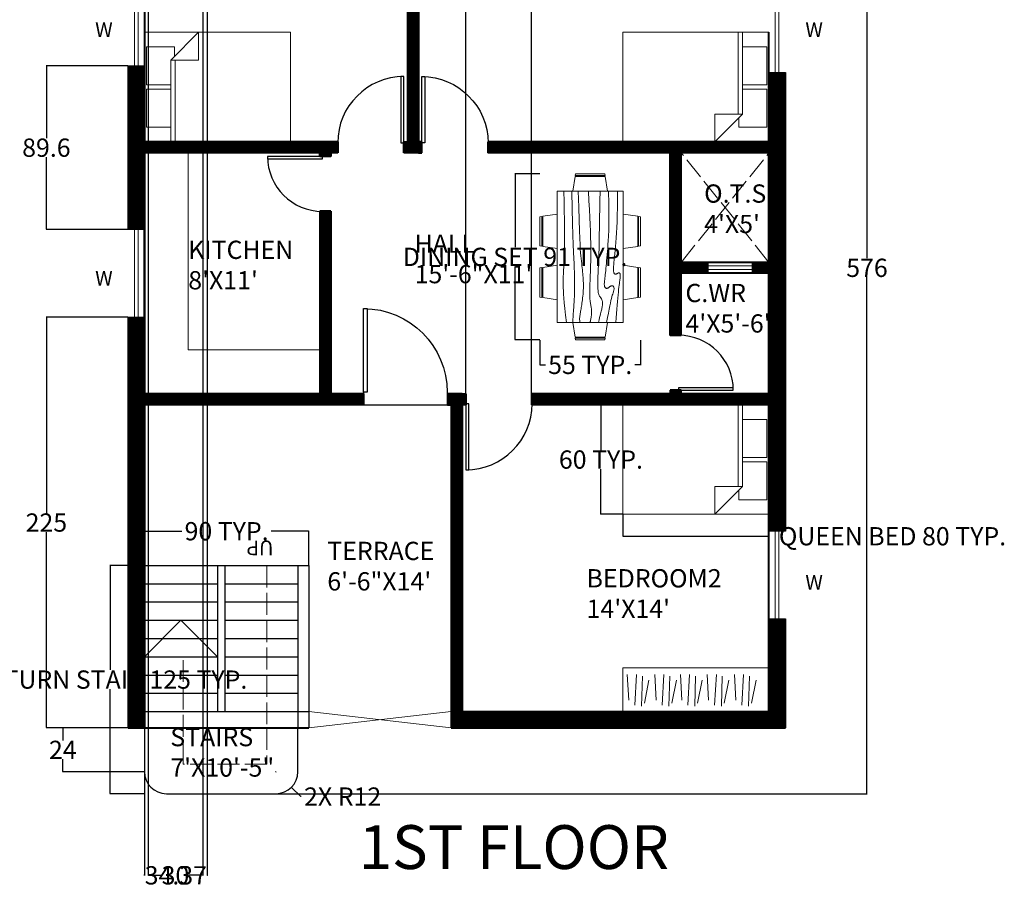
# Model space of a CAD drawing. Units: inches. Extents: x 345 to 1363, y 285 to 1014.
# Tile 3 of 4: x 824 to 1363, y 285 to 760. Entities that reach past the tile are written whole.
import ezdxf

# ---------------------------------------------------------------- set-up
doc = ezdxf.new("R2010")
doc.units = ezdxf.units.IN
doc.header["$MEASUREMENT"] = 0
doc.linetypes.add('ACAD_ISO02W100', pattern=[15, 12, -3])
for name, color, linetype, lineweight in [('A-ANNO-DIMS', 2, 'Continuous', 18), ('A-ANNO-SYMB', 3, 'Continuous', 18), ('A-ANNO-TEXT', 7, 'Continuous', 18), ('A-ANNO-TITL', 7, 'Continuous', 35), ('A-AREA-IDEN', 7, 'Continuous', 18), ('A-FLOR-CASE', 8, 'Continuous', 18), ('A-FLOR-OPEN', 8, 'Continuous', 18), ('A-FLOR-OPEN-OVHD', 8, 'ACAD_ISO02W100', 13), ('A-FLOR-STRS', 7, 'Continuous', 25), ('A-FLOR-STRS-PATH', 3, 'ACAD_ISO02W100', 18), ('A-FURN', 9, 'Continuous', 18), ('A-GLAZ', 4, 'Continuous', 18), ('A-WALL', 7, 'Continuous', 40), ('A-WALL-PATT', 252, 'Continuous', 9), ('BED', 9, 'Continuous', 18), ('DOOR', 4, 'Continuous', 25)]:
    doc.layers.add(name, color=color, linetype=linetype, lineweight=lineweight)
doc.styles.get("Standard").update_dxf_attribs({"font": 'arial.ttf'})
doc.dimstyles.get("Standard").update_dxf_attribs({"dimtxt": 10, "dimasz": 0.18, "dimexe": 0.18, "dimexo": 0.0625, "dimgap": 0.09, "dimtad": 0, "dimtih": 1, "dimtoh": 1, "dimdec": 0, "dimzin": 0, "dimdsep": 46, "dimlunit": 3, "dimtxsty": 'Standard', "dimcen": 0.09, "dimadec": 0, "dimazin": 0, "dimtfac": 1, "dimtdec": 0, "dimtofl": 0, "dimtmove": 0, "dimatfit": 3, "dimfxl": 1, "dimtolj": 1, "dimtzin": 0, "dimarcsym": 0})

# ---------------------------------------------------------------- blocks, each defined once
blk = doc.blocks.new('Bed - Queen')
for p, q in [((0, -80.00003), (0, 0)), ((0, 0), (59.99999, 0)), ((59.99999, 0), (59.99999, -80.00003)), ((7.99999, -1.2), (28.79998, -1.2)), ((7.99999, -14.4), (7.99999, -1.2)), ((28.79998, -1.2), (28.79998, -14.4)), ((31.19999, -1.2), (51.99999, -1.2)), ((31.19999, -14.4), (31.19999, -1.2)), ((51.99999, -1.2), (51.99999, -16.4)), ((0, -14.4), (44.8, -14.4)), ((59.99999, -29.6), (44.8, -14.4)), ((44.8, -14.4), (44.8, -29.6)), ((44.8, -16.8), (0, -16.8)), ((51.99999, -16.4), (46.79936, -16.4)), ((44.8, -29.6), (59.99999, -29.6)), ((59.99999, -80.00003), (0, -80.00003))]:
    blk.add_line(p, q)
blk = doc.blocks.new('Dining Set - 36 x 72 in.')
for p, q in [((-22, 27.5), (-22.1562, 26.50042)), ((-22, 27.5), (-6, 27.5)), ((-5.8437, 26.49966), (-6, 27.5)), ((6, 27.5), (5.8438, 26.50042)), ((6, 27.5), (22, 27.5)), ((22.1563, 26.49966), (22, 27.5)), ((-22.2343, 26.00059), (-23.4847, 17.99762)), ((-22.2304, 26), (-5.7608, 26)), ((-5.8416, 26.5), (-22.1534, 26.5)), ((-4.5152, 17.99762), (-5.7655, 25.99926)), ((5.7657, 26.00059), (4.5153, 17.99762)), ((5.7696, 26), (22.2392, 26)), ((22.1584, 26.5), (5.8466, 26.5)), ((23.4848, 17.99762), (22.2345, 25.99926)), ((36, 18), (-36, 18)), ((-36, 18), (-36, -18)), ((36, -18), (36, 18)), ((-45.5, 8), (-44.5004, 8.15617)), ((-45.5, 8), (-45.5, -8)), ((-44.5, -8.15843), (-44.5, 8.15338)), ((-44.0006, 8.23428), (-35.9976, 9.48474)), ((-44, 8.23041), (-44, -8.23915)), ((44.0006, 8.23428), (35.9976, 9.48474)), ((44, 8.23041), (44, -8.23915)), ((44.5, -8.15843), (44.5, 8.15338)), ((45.5, 8), (44.5005, 8.15617)), ((45.5, 8), (45.5, -8)), ((-44.4997, -8.15631), (-45.5, -8)), ((-35.9976, -9.48476), (-43.9993, -8.2345)), ((35.9976, -9.48476), (43.9993, -8.2345)), ((44.4997, -8.15631), (45.5, -8)), ((-36, -18), (36, -18)), ((-22.2343, -26.0006), (-23.4847, -17.99762)), ((-4.5152, -17.99762), (-5.7655, -25.99928)), ((5.7657, -26.0006), (4.5153, -17.99762)), ((23.4848, -17.99762), (22.2345, -25.99928)), ((-22.2304, -26), (-5.7608, -26)), ((-22, -27.5), (-22.1562, -26.50044)), ((-5.8416, -26.5), (-22.1534, -26.5)), ((-5.8437, -26.49967), (-6, -27.5)), ((5.7696, -26), (22.2392, -26)), ((6, -27.5), (5.8438, -26.50044)), ((22.1584, -26.5), (5.8466, -26.5)), ((22.1563, -26.49967), (22, -27.5)), ((-22, -27.5), (-6, -27.5)), ((6, -27.5), (22, -27.5))]:
    blk.add_line(p, q)
for points in [[(-36, 15), (-31.1772, 14.97754), (-26.8079, 14.91406), (-22.8538, 14.81543), (-19.276, 14.6875), (-16.0362, 14.53613), (-13.0957, 14.36718), (-10.4159, 14.18652), (-7.9583, 14), (-5.6904, 13.81315), (-3.6035, 13.63021), (-1.6954, 13.45508), (0.0365, 13.29166), (1.5945, 13.14388), (2.9811, 13.01562), (4.1988, 12.9108), (5.25, 12.83333), (6.1393, 12.78613), (6.8802, 12.76823), (7.4883, 12.77767), (7.9792, 12.8125), (8.3685, 12.87077), (8.6719, 12.95052), (8.9049, 13.0498), (9.0833, 13.16666), (9.2205, 13.29899), (9.3216, 13.44401), (9.3895, 13.59879), (9.4271, 13.76041), (9.4373, 13.92594), (9.4232, 14.09245), (9.3875, 14.257), (9.3333, 14.41666), (9.2638, 14.56917), (9.1836, 14.71484), (9.0975, 14.85465), (9.0104, 14.98958), (8.9272, 15.1206), (8.8529, 15.2487), (8.7922, 15.37483), (8.75, 15.5), (8.7305, 15.62467), (8.7344, 15.74739), (8.7617, 15.86621), (8.8125, 15.97916), (8.8867, 16.08431), (8.9844, 16.17968), (9.1055, 16.26334), (9.25, 16.33333), (9.4189, 16.38802), (9.6172, 16.42708), (9.8506, 16.45052), (10.125, 16.45833), (10.4463, 16.45052), (10.8203, 16.42708), (11.2529, 16.38802), (11.75, 16.33333), (12.3184, 16.26318), (12.9694, 16.17838), (13.7151, 16.07991), (14.5677, 15.96875), (15.5395, 15.84586), (16.6426, 15.71224), (17.8893, 15.56884), (19.2917, 15.41666), (20.859, 15.25667), (22.5879, 15.08984), (24.4721, 14.91715), (26.5052, 14.73958), (28.6809, 14.5581), (30.9929, 14.3737), (33.4347, 14.18733), (36, 14)], [(-36, 10), (-28.9766, 10.14274), (-23.1725, 10.20442), (-18.4241, 10.19775), (-14.5677, 10.13541), (-11.4399, 10.03011), (-8.877, 9.89453), (-6.7154, 9.74137), (-4.7917, 9.58333), (-2.9698, 9.43082), (-1.2246, 9.28515), (0.4415, 9.14534), (2.026, 9.01041), (3.5266, 8.87939), (4.9408, 8.7513), (6.266, 8.62516), (7.5, 8.5), (8.6411, 8.37549), (9.6914, 8.2539), (10.6538, 8.13818), (11.5312, 8.03125), (12.3267, 7.93603), (13.043, 7.85547), (13.6831, 7.79248), (14.25, 7.75), (14.7471, 7.7303), (15.1797, 7.73307), (15.5537, 7.75732), (15.875, 7.80208), (16.1494, 7.86637), (16.3828, 7.94922), (16.5811, 8.04964), (16.75, 8.16666), (16.8944, 8.29915), (17.0143, 8.44531), (17.1089, 8.60319), (17.1771, 8.77083), (17.218, 8.94629), (17.2305, 9.1276), (17.2137, 9.31282), (17.1667, 9.5), (17.0895, 9.6875), (16.987, 9.875), (16.8649, 10.0625), (16.7292, 10.25), (16.5856, 10.4375), (16.4401, 10.625), (16.2985, 10.8125), (16.1667, 11), (16.05, 11.18733), (15.9518, 11.3737), (15.8752, 11.5581), (15.8229, 11.73958), (15.798, 11.91715), (15.8034, 12.08984), (15.842, 12.25667), (15.9167, 12.41666), (16.0295, 12.56836), (16.1784, 12.70833), (16.3605, 12.83268), (16.5729, 12.9375), (16.8127, 13.01888), (17.0768, 13.07291), (17.3625, 13.0957), (17.6667, 13.08333), (17.9894, 13.03312), (18.3418, 12.94726), (18.7382, 12.82918), (19.1927, 12.68229), (19.7195, 12.51001), (20.3327, 12.31575), (21.0465, 12.10294), (21.875, 11.875), (22.8357, 11.63354), (23.959, 11.37304), (25.2786, 11.08618), (26.8282, 10.76562), (28.6414, 10.40405), (30.752, 9.99414), (33.1936, 9.52856), (36, 9)], [(-36, 5.5), (-30.7157, 5.3348), (-26.069, 5.20963), (-21.9946, 5.11767), (-18.4271, 5.05208), (-15.3009, 5.00602), (-12.5508, 4.97265), (-10.1112, 4.94515), (-7.9167, 4.91666), (-5.909, 4.88167), (-4.0586, 4.83984), (-2.3429, 4.79215), (-0.7396, 4.73958), (0.7739, 4.6831), (2.22, 4.6237), (3.6213, 4.56233), (5, 4.5), (6.373, 4.43782), (7.7344, 4.3776), (9.0723, 4.32129), (10.375, 4.27083), (11.6309, 4.22819), (12.8281, 4.19531), (13.9551, 4.17415), (15, 4.16666), (15.954, 4.17448), (16.819, 4.19791), (17.6001, 4.23698), (18.3021, 4.29166), (18.9299, 4.36198), (19.4883, 4.44791), (19.9823, 4.54948), (20.4167, 4.66666), (20.7969, 4.79899), (21.1302, 4.94401), (21.4245, 5.09879), (21.6875, 5.26041), (21.9271, 5.42594), (22.1511, 5.59245), (22.3672, 5.757), (22.5834, 5.91666), (22.8065, 6.06868), (23.0404, 6.21093), (23.2879, 6.34147), (23.5521, 6.45833), (23.8358, 6.55957), (24.142, 6.64323), (24.4735, 6.70735), (24.8334, 6.75), (25.2235, 6.76969), (25.642, 6.76692), (26.0858, 6.74267), (26.5521, 6.69791), (27.0379, 6.63362), (27.5404, 6.55078), (28.0565, 6.45036), (28.5834, 6.33333), (29.1242, 6.19987), (29.7071, 6.04687), (30.3661, 5.87044), (31.1354, 5.66666), (32.0493, 5.43164), (33.142, 5.16146), (34.4475, 4.85221), (36, 4.5)], [(-36, -1), (-30.7915, -0.6591), (-26.0195, -0.38216), (-21.6519, -0.16284), (-17.6563, 0.00521), (-14.0005, 0.12833), (-10.6523, 0.21289), (-7.5796, 0.26522), (-4.75, 0.29166), (-2.134, 0.29793), (0.2878, 0.28711), (2.5317, 0.26163), (4.6146, 0.22396), (6.5529, 0.17651), (8.3633, 0.12174), (10.0623, 0.06209), (11.6667, 0), (13.1899, -0.06201), (14.6341, -0.1211), (15.9982, -0.17432), (17.2813, -0.21875), (18.4823, -0.25147), (19.6003, -0.26953), (20.6343, -0.27002), (21.5834, -0.25), (22.4481, -0.20768), (23.2357, -0.14584), (23.9549, -0.06836), (24.6146, 0.02083), (25.2235, 0.11784), (25.7904, 0.21875), (26.3241, 0.31966), (26.8334, 0.41666), (27.3265, 0.50618), (27.8099, 0.58593), (28.2894, 0.65397), (28.7709, 0.70833), (29.2601, 0.74707), (29.763, 0.76823), (30.2855, 0.76985), (30.8334, 0.75), (31.4088, 0.70784), (31.9994, 0.64713), (32.589, 0.57275), (33.1615, 0.48958), (33.7008, 0.4025), (34.1908, 0.3164), (34.6153, 0.23616), (34.9584, 0.16666), (35.2099, 0.11165), (35.3848, 0.07031), (35.504, 0.04069), (35.5886, 0.02083), (35.6594, 0.00879), (35.7377, 0.0026), (35.8442, 0.00032), (36, 0)], [(-36, -6.5), (-27.1843, -6.31267), (-20.084, -6.1263), (-14.469, -5.9419), (-10.1094, -5.76042), (-6.7752, -5.58285), (-4.2363, -5.41016), (-2.2629, -5.24333), (-0.625, -5.08334), (0.8708, -4.93099), (2.2715, -4.78646), (3.5872, -4.64974), (4.8281, -4.52084), (6.0046, -4.39974), (7.127, -4.28646), (8.2053, -4.18099), (9.25, -4.08334), (10.2705, -3.99382), (11.2734, -3.91407), (12.2647, -3.84603), (13.25, -3.79167), (14.2354, -3.75293), (15.2266, -3.73177), (16.2295, -3.73015), (17.25, -3.75), (18.2912, -3.79248), (19.3451, -3.85547), (20.4009, -3.93604), (21.4479, -4.03125), (22.4754, -4.13819), (23.4727, -4.25391), (24.4289, -4.37549), (25.3334, -4.5), (26.1785, -4.62492), (26.9694, -4.74935), (27.7145, -4.87281), (28.4219, -4.99479), (29.1, -5.11483), (29.7572, -5.23242), (30.4016, -5.34709), (31.0417, -5.45834), (31.6837, -5.56437), (32.3262, -5.65821), (32.9658, -5.73153), (33.599, -5.77604), (34.2224, -5.78345), (34.8327, -5.74545), (35.4264, -5.65373), (36, -5.5)], [(-36, -10), (-26.4022, -9.81299), (-18.4675, -9.62891), (-11.9839, -9.45069), (-6.7396, -9.28125), (-2.5226, -9.12354), (0.8789, -8.98047), (3.6769, -8.85498), (6.0833, -8.75), (8.2767, -8.66765), (10.3021, -8.60677), (12.1712, -8.56543), (13.8958, -8.54167), (15.4876, -8.53353), (16.9583, -8.53907), (18.3197, -8.55632), (19.5834, -8.58334), (20.7616, -8.61841), (21.8685, -8.66081), (22.9188, -8.71004), (23.9271, -8.76563), (24.9081, -8.82707), (25.8763, -8.89388), (26.8465, -8.96558), (27.8334, -9.04167), (28.8474, -9.12118), (29.8828, -9.20117), (30.93, -9.27824), (31.9792, -9.34896), (33.0205, -9.40991), (34.0443, -9.45768), (35.0407, -9.48885), (36, -9.5)], [(-36, -14.5), (-30.0881, -14.33513), (-25.0332, -14.21224), (-20.7312, -14.12647), (-17.0781, -14.07292), (-13.97, -14.04671), (-11.3027, -14.04297), (-8.9724, -14.05681), (-6.875, -14.08334), (-4.9224, -14.11833), (-3.0905, -14.16016), (-1.3709, -14.20785), (0.2448, -14.26042), (1.7647, -14.3169), (3.1973, -14.3763), (4.5507, -14.43767), (5.8333, -14.5), (7.0554, -14.5621), (8.235, -14.62175), (9.3922, -14.67652), (10.5469, -14.72396), (11.7192, -14.76164), (12.929, -14.78711), (14.1965, -14.79794), (15.5417, -14.79167), (16.9933, -14.76424), (18.6152, -14.70508), (20.4804, -14.60197), (22.6615, -14.44271), (25.2312, -14.21509), (28.2624, -13.9069), (31.8277, -13.50594), (36, -13)]]:
    blk.add_lwpolyline(points)
blk = doc.blocks.new('*U8')
for p, q in [((0, 0), (0, -6)), ((-40, 0), (-40, -6))]:
    blk.add_line(p, q)
blk.add_lwpolyline([(0, 0), (0, 40), (-1.75, 40), (-1.75, 0)], close=True)
blk.add_arc((0, 0), 40, 90, 180)
blk = doc.blocks.new('*U9')
for p, q in [((0, 0), (0, 6)), ((40, 0), (40, 6))]:
    blk.add_line(p, q)
blk.add_lwpolyline([(0, 0), (0, -40), (1.75, -40), (1.75, 0)], close=True)
blk.add_arc((0, 0), 40, 270, 360)
blk = doc.blocks.new('WIN-48IN-EXT')
for p, q in [((9, 48), (0, 48)), ((3.5, 0), (3.5, 48)), ((5.5, 0), (5.5, 48)), ((9, 0), (0, 0))]:
    blk.add_line(p, q)
blk = doc.blocks.new('WIN-24IN-VENT')
for p, q in [((0, 24), (6, 24)), ((2, 24), (2, 0)), ((4, 24), (4, 0)), ((0, 0), (6, 0))]:
    blk.add_line(p, q)
blk = doc.blocks.new('WARDROBE-80X24')
for p, q in [((0, 0), (0, 24)), ((80, 0), (80, 24)), ((2.45, 20.28), (3.21, 6.18)), ((7.49, 20.28), (6.48, 3.41)), ((10.77, 19.28), (10.26, 2.91)), ((14.3, 17.26), (11.77, 4.67)), ((17.45, 20.28), (18.2, 6.18)), ((22.49, 20.28), (21.48, 3.41)), ((25.77, 19.28), (25.26, 2.91)), ((29.29, 17.26), (26.77, 4.67)), ((31.55, 20.28), (32.31, 6.18)), ((36.59, 20.28), (35.59, 3.41)), ((39.87, 19.28), (39.37, 2.91)), ((43.4, 17.26), (40.88, 4.67)), ((46.16, 20.28), (46.91, 6.18)), ((51.2, 20.28), (50.19, 3.41)), ((54.47, 19.28), (53.97, 2.91)), ((58, 17.26), (55.48, 4.67)), ((61.07, 20.28), (61.83, 6.18)), ((66.11, 20.28), (65.1, 3.41)), ((69.39, 19.28), (68.88, 2.91)), ((72.92, 17.26), (70.4, 4.67)), ((80, 0), (0, 0))]:
    blk.add_line(p, q)
blk = doc.blocks.new('KITCHEN-L-COUNTER')
for p in [(0, 108), (72, 0)]:
    blk.add_line(p, (0, 0))
blk = doc.blocks.new('STAIR-RETURN-84IN')
for p, q in [((0, 89), (44, 89)), ((40, 89), (40, 9)), ((44, 89), (44, 9)), ((44, 89), (90, 89)), ((84, 89), (84, 0)), ((90, 89), (90, 0)), ((0, 79), (40, 79)), ((44, 79), (84, 79)), ((0, 69), (40, 69)), ((44, 69), (84, 69)), ((0, 59), (40, 59)), ((44, 59), (84, 59)), ((0, 49), (40, 49)), ((44, 49), (84, 49)), ((0, 39), (40, 39)), ((44, 39), (84, 39)), ((0, 29), (40, 29)), ((44, 29), (84, 29)), ((0, 19), (40, 19)), ((44, 19), (84, 19)), ((0, 9), (90, 9)), ((0, 0), (0, -24)), ((84, -24), (84, 0)), ((12, -36), (72, -36))]:
    blk.add_line(p, q)
for centre, start, end in [((12, -24), 180, 270), ((72, -24), 270, 0)]:
    blk.add_arc(centre, 12, start, end)
blk = doc.blocks.new('STAIR-DIRECTION-ARROWHEAD')
for p, q in [((-20, 0), (0, 20)), ((0, 20), (20, 0)), ((0, 0), (-20, 0)), ((20, 0), (1.17, 0))]:
    blk.add_line(p, q)
blk = doc.blocks.new('*D20')
at = {"layer": 'A-ANNO-DIMS', "color": 0, "lineweight": -2, "transparency": 16777216}
for p, q in [((1154.38, 488.7), (1154.38, 476.58)), ((1234.38, 488.7), (1234.38, 476.58)), ((1154.56, 476.76), (1234.2, 476.76)), ((1234.38, 476.76), (1234.56, 476.76))]:
    blk.add_line(p, q, dxfattribs=at)
at = {"layer": 'A-ANNO-DIMS', "color": 0, "transparency": 16777216}
for points in [[(1154.56, 476.79), (1154.56, 476.73), (1154.38, 476.76)], [(1234.2, 476.79), (1234.2, 476.73), (1234.38, 476.76)]]:
    blk.add_solid(points, dxfattribs=at)
at = {"layer": 'Defpoints', "color": 0, "transparency": 16777216}
for p in [(1154.38, 488.76), (1234.38, 488.76), (1234.38, 476.76)]:
    blk.add_point(p, dxfattribs=at)
at = {"layer": 'A-ANNO-DIMS', "color": 0, "transparency": 16777216, "insert": (1302.06, 476.76), "char_height": 10, "attachment_point": 5}
blk.add_mtext('\\A1;QUEEN BED 80 TYP.', dxfattribs=at)
blk = doc.blocks.new('*D21')
at = {"layer": 'A-ANNO-DIMS', "color": 0, "lineweight": -2, "transparency": 16777216}
for p, q in [((1154.32, 548.76), (1142.2, 548.76)), ((1142.38, 548.58), (1142.38, 523.96)), ((1142.38, 488.94), (1142.38, 513.57)), ((1154.32, 488.76), (1142.2, 488.76))]:
    blk.add_line(p, q, dxfattribs=at)
at = {"layer": 'A-ANNO-DIMS', "color": 0, "transparency": 16777216}
for points in [[(1142.35, 548.58), (1142.41, 548.58), (1142.38, 548.76)], [(1142.35, 488.94), (1142.41, 488.94), (1142.38, 488.76)]]:
    blk.add_solid(points, dxfattribs=at)
at = {"layer": 'Defpoints', "color": 0, "transparency": 16777216}
for p in [(1154.38, 548.76), (1142.38, 488.76), (1154.38, 488.76)]:
    blk.add_point(p, dxfattribs=at)
at = {"layer": 'A-ANNO-DIMS', "color": 0, "transparency": 16777216, "insert": (1142.38, 518.76), "char_height": 10, "attachment_point": 5}
blk.add_mtext('\\A1;60 TYP.', dxfattribs=at)
blk = doc.blocks.new('*D24')
at = {"layer": 'A-ANNO-DIMS', "color": 0, "lineweight": -2, "transparency": 16777216}
for p, q in [((1108.94, 675.25), (1095.17, 675.25)), ((1095.35, 675.07), (1095.35, 635.01)), ((1095.35, 584.43), (1095.35, 624.48)), ((1108.94, 584.25), (1095.17, 584.25))]:
    blk.add_line(p, q, dxfattribs=at)
at = {"layer": 'A-ANNO-DIMS', "color": 0, "transparency": 16777216}
for points in [[(1095.32, 675.07), (1095.38, 675.07), (1095.35, 675.25)], [(1095.32, 584.43), (1095.38, 584.43), (1095.35, 584.25)]]:
    blk.add_solid(points, dxfattribs=at)
at = {"layer": 'Defpoints', "color": 0, "transparency": 16777216}
for p in [(1109, 675.25), (1095.35, 584.25), (1109, 584.25)]:
    blk.add_point(p, dxfattribs=at)
at = {"layer": 'A-ANNO-DIMS', "color": 0, "transparency": 16777216, "insert": (1095.35, 629.75), "char_height": 10, "attachment_point": 5}
blk.add_mtext('\\A1;DINING SET 91 TYP.', dxfattribs=at)
blk = doc.blocks.new('*D25')
at = {"layer": 'A-ANNO-DIMS', "color": 0, "lineweight": -2, "transparency": 16777216}
for p, q in [((1109, 584.18), (1109, 570.42)), ((1164, 584.18), (1164, 570.42)), ((1109.18, 570.6), (1112.07, 570.6)), ((1163.82, 570.6), (1160.93, 570.6))]:
    blk.add_line(p, q, dxfattribs=at)
at = {"layer": 'A-ANNO-DIMS', "color": 0, "transparency": 16777216}
for points in [[(1109.18, 570.63), (1109.18, 570.57), (1109, 570.6)], [(1163.82, 570.63), (1163.82, 570.57), (1164, 570.6)]]:
    blk.add_solid(points, dxfattribs=at)
at = {"layer": 'Defpoints', "color": 0, "transparency": 16777216}
for p in [(1109, 584.25), (1164, 584.25), (1164, 570.6)]:
    blk.add_point(p, dxfattribs=at)
at = {"layer": 'A-ANNO-DIMS', "color": 0, "transparency": 16777216, "insert": (1136.5, 570.6), "char_height": 10, "attachment_point": 5}
blk.add_mtext('\\A1;55 TYP.', dxfattribs=at)
blk = doc.blocks.new('*D28')
at = {"layer": 'A-ANNO-DIMS', "color": 0, "lineweight": -2, "transparency": 16777216}
for p, q in [((892.32, 460.76), (873.45, 460.76)), ((873.63, 460.58), (873.63, 403.52)), ((873.63, 335.94), (873.63, 393)), ((892.32, 335.76), (873.45, 335.76))]:
    blk.add_line(p, q, dxfattribs=at)
at = {"layer": 'A-ANNO-DIMS', "color": 0, "transparency": 16777216}
for points in [[(873.6, 460.58), (873.66, 460.58), (873.63, 460.76)], [(873.6, 335.94), (873.66, 335.94), (873.63, 335.76)]]:
    blk.add_solid(points, dxfattribs=at)
at = {"layer": 'Defpoints', "color": 0, "transparency": 16777216}
for p in [(873.63, 460.76), (892.38, 460.76), (892.38, 335.76)]:
    blk.add_point(p, dxfattribs=at)
at = {"layer": 'A-ANNO-DIMS', "color": 0, "transparency": 16777216, "insert": (873.63, 398.26), "char_height": 10, "attachment_point": 5}
blk.add_mtext('\\A1;RETURN STAIR 125 TYP.', dxfattribs=at)
blk = doc.blocks.new('*D29')
at = {"layer": 'A-ANNO-DIMS', "color": 0, "lineweight": -2, "transparency": 16777216}
for p, q in [((892.38, 460.83), (892.38, 479.69)), ((892.56, 479.51), (912.95, 479.51)), ((982.2, 479.51), (961.81, 479.51)), ((982.38, 460.83), (982.38, 479.69))]:
    blk.add_line(p, q, dxfattribs=at)
at = {"layer": 'A-ANNO-DIMS', "color": 0, "transparency": 16777216}
for points in [[(892.56, 479.54), (892.56, 479.48), (892.38, 479.51)], [(982.2, 479.54), (982.2, 479.48), (982.38, 479.51)]]:
    blk.add_solid(points, dxfattribs=at)
at = {"layer": 'Defpoints', "color": 0, "transparency": 16777216}
for p in [(982.38, 479.51), (892.38, 460.76), (982.38, 460.76)]:
    blk.add_point(p, dxfattribs=at)
at = {"layer": 'A-ANNO-DIMS', "color": 0, "transparency": 16777216, "insert": (937.38, 479.51), "char_height": 10, "attachment_point": 5}
blk.add_mtext('\\A1;90 TYP.', dxfattribs=at)
blk = doc.blocks.new('*D33')
at = {"layer": 'A-ANNO-DIMS', "color": 0, "lineweight": -2, "transparency": 16777216}
for p, q in [((1243.44, 911.76), (1288.26, 911.76)), ((1288.08, 911.58), (1288.08, 628.96)), ((1288.08, 335.94), (1288.08, 618.57)), ((964.44, 335.76), (1288.26, 335.76))]:
    blk.add_line(p, q, dxfattribs=at)
at = {"layer": 'A-ANNO-DIMS', "color": 0, "transparency": 16777216}
for points in [[(1288.05, 911.58), (1288.11, 911.58), (1288.08, 911.76)], [(1288.05, 335.94), (1288.11, 335.94), (1288.08, 335.76)]]:
    blk.add_solid(points, dxfattribs=at)
at = {"layer": 'Defpoints', "color": 0, "transparency": 16777216}
for p in [(1243.38, 911.76), (1288.08, 911.76), (964.38, 335.76)]:
    blk.add_point(p, dxfattribs=at)
at = {"layer": 'A-ANNO-DIMS', "color": 0, "transparency": 16777216, "insert": (1288.08, 623.76), "char_height": 10, "attachment_point": 5}
blk.add_mtext('\\A1;576', dxfattribs=at)
blk = doc.blocks.new('*D34')
at = {"layer": 'A-ANNO-DIMS', "color": 0, "lineweight": -2, "transparency": 16777216}
for p, q in [((883.32, 596.76), (838.5, 596.76)), ((838.68, 596.58), (838.68, 489.46)), ((838.68, 371.94), (838.68, 479.07)), ((883.32, 371.76), (838.5, 371.76))]:
    blk.add_line(p, q, dxfattribs=at)
at = {"layer": 'A-ANNO-DIMS', "color": 0, "transparency": 16777216}
for points in [[(838.65, 596.58), (838.71, 596.58), (838.68, 596.76)], [(838.65, 371.94), (838.71, 371.94), (838.68, 371.76)]]:
    blk.add_solid(points, dxfattribs=at)
at = {"layer": 'Defpoints', "color": 0, "transparency": 16777216}
for p in [(838.68, 596.76), (883.38, 596.76), (883.38, 371.76)]:
    blk.add_point(p, dxfattribs=at)
at = {"layer": 'A-ANNO-DIMS', "color": 0, "transparency": 16777216, "insert": (838.68, 484.26), "char_height": 10, "attachment_point": 5}
blk.add_mtext('\\A1;225', dxfattribs=at)
blk = doc.blocks.new('*D35')
at = {"layer": 'A-ANNO-DIMS', "color": 0, "lineweight": -2, "transparency": 16777216}
for p, q in [((883.32, 734.36), (838.5, 734.36)), ((838.68, 734.18), (838.68, 694.76)), ((838.68, 644.94), (838.68, 684.37)), ((883.32, 644.76), (838.5, 644.76))]:
    blk.add_line(p, q, dxfattribs=at)
at = {"layer": 'A-ANNO-DIMS', "color": 0, "transparency": 16777216}
for points in [[(838.65, 734.18), (838.71, 734.18), (838.68, 734.36)], [(838.65, 644.94), (838.71, 644.94), (838.68, 644.76)]]:
    blk.add_solid(points, dxfattribs=at)
at = {"layer": 'Defpoints', "color": 0, "transparency": 16777216}
for p in [(838.68, 734.36), (883.38, 734.36), (883.38, 644.76)]:
    blk.add_point(p, dxfattribs=at)
at = {"layer": 'A-ANNO-DIMS', "color": 0, "transparency": 16777216, "insert": (838.68, 689.56), "char_height": 10, "attachment_point": 5}
blk.add_mtext('\\A1;89.6', dxfattribs=at)
blk = doc.blocks.new('*D36')
at = {"layer": 'A-ANNO-DIMS', "color": 0, "lineweight": -2, "transparency": 16777216}
for p, q in [((892.32, 371.76), (847.5, 371.76)), ((847.68, 371.58), (847.68, 364.87)), ((847.68, 347.94), (847.68, 354.65)), ((892.32, 347.76), (847.5, 347.76))]:
    blk.add_line(p, q, dxfattribs=at)
at = {"layer": 'A-ANNO-DIMS', "color": 0, "transparency": 16777216}
for points in [[(847.65, 371.58), (847.71, 371.58), (847.68, 371.76)], [(847.65, 347.94), (847.71, 347.94), (847.68, 347.76)]]:
    blk.add_solid(points, dxfattribs=at)
at = {"layer": 'Defpoints', "color": 0, "transparency": 16777216}
for p in [(847.68, 371.76), (892.38, 371.76), (892.38, 347.76)]:
    blk.add_point(p, dxfattribs=at)
at = {"layer": 'A-ANNO-DIMS', "color": 0, "transparency": 16777216, "insert": (847.68, 359.76), "char_height": 10, "attachment_point": 5}
blk.add_mtext('\\A1;24', dxfattribs=at)
blk = doc.blocks.new('*D41')
at = {"layer": 'A-ANNO-DIMS', "color": 0, "lineweight": -2, "transparency": 16777216}
for p, q in [((894.38, 824.7), (894.38, 290.88)), ((924.38, 824.7), (924.38, 290.88)), ((894.56, 291.06), (902.15, 291.06)), ((924.2, 291.06), (916.61, 291.06))]:
    blk.add_line(p, q, dxfattribs=at)
at = {"layer": 'A-ANNO-DIMS', "color": 0, "transparency": 16777216}
for points in [[(894.56, 291.09), (894.56, 291.03), (894.38, 291.06)], [(924.2, 291.09), (924.2, 291.03), (924.38, 291.06)]]:
    blk.add_solid(points, dxfattribs=at)
at = {"layer": 'Defpoints', "color": 0, "transparency": 16777216}
for p in [(894.38, 824.76), (924.38, 824.76), (924.38, 291.06)]:
    blk.add_point(p, dxfattribs=at)
at = {"layer": 'A-ANNO-DIMS', "color": 0, "transparency": 16777216, "insert": (909.38, 291.06), "char_height": 10, "attachment_point": 5}
blk.add_mtext('\\A1;30', dxfattribs=at)
blk = doc.blocks.new('*D42')
at = {"layer": 'A-ANNO-DIMS', "color": 0, "lineweight": -2, "transparency": 16777216}
for p, q in [((1068.38, 554.83), (1068.38, 1007.64)), ((1068.56, 1007.46), (1079.14, 1007.46)), ((1104.2, 1007.46), (1093.63, 1007.46)), ((1104.38, 554.83), (1104.38, 1007.64))]:
    blk.add_line(p, q, dxfattribs=at)
at = {"layer": 'A-ANNO-DIMS', "color": 0, "transparency": 16777216}
for points in [[(1068.56, 1007.49), (1068.56, 1007.43), (1068.38, 1007.46)], [(1104.2, 1007.49), (1104.2, 1007.43), (1104.38, 1007.46)]]:
    blk.add_solid(points, dxfattribs=at)
at = {"layer": 'Defpoints', "color": 0, "transparency": 16777216}
for p in [(1104.38, 1007.46), (1068.38, 554.76), (1104.38, 554.76)]:
    blk.add_point(p, dxfattribs=at)
at = {"layer": 'A-ANNO-DIMS', "color": 0, "transparency": 16777216, "insert": (1086.38, 1007.46), "char_height": 10, "attachment_point": 5}
blk.add_mtext('\\A1;36', dxfattribs=at)
blk = doc.blocks.new('*D46')
at = {"layer": 'A-ANNO-DIMS', "color": 0, "lineweight": -2, "transparency": 16777216}
for p, q in [((892.381853, 902.701559), (892.381853, 290.884059)), ((926.755051, 894.701559), (926.755051, 290.884059)), ((892.201853, 291.064059), (892.021853, 291.064059)), ((926.935051, 291.064059), (927.115051, 291.064059))]:
    blk.add_line(p, q, dxfattribs=at)
at = {"layer": 'A-ANNO-DIMS', "color": 0, "transparency": 16777216}
for points in [[(892.201853, 291.094059), (892.201853, 291.034059), (892.381853, 291.064059)], [(926.935051, 291.094059), (926.935051, 291.034059), (926.755051, 291.064059)]]:
    blk.add_solid(points, dxfattribs=at)
at = {"layer": 'Defpoints', "color": 0, "transparency": 16777216}
for p in [(892.381853, 902.764059), (926.755051, 894.764059), (926.755051, 291.064059)]:
    blk.add_point(p, dxfattribs=at)
at = {"layer": 'A-ANNO-DIMS', "color": 0, "transparency": 16777216, "insert": (909.568452, 291.064059), "char_height": 10, "attachment_point": 5}
blk.add_mtext('\\A1;34.37', dxfattribs=at)
blk = doc.blocks.new('*D48')
at = {"layer": 'A-ANNO-DIMS', "color": 0, "lineweight": -2, "transparency": 16777216}
for p, q in [((964.29, 347.76), (964.47, 347.76)), ((964.38, 347.67), (964.38, 347.85)), ((977.96, 334.19), (972.99, 339.15)), ((978.14, 334.19), (977.96, 334.19))]:
    blk.add_line(p, q, dxfattribs=at)
at = {"layer": 'A-ANNO-DIMS', "color": 0, "transparency": 16777216}
blk.add_solid([(973.02, 339.17), (972.97, 339.13), (972.87, 339.28)], dxfattribs=at)
at = {"layer": 'Defpoints', "color": 0, "transparency": 16777216}
for p in [(964.38, 347.76), (972.87, 339.28)]:
    blk.add_point(p, dxfattribs=at)
at = {"layer": 'A-ANNO-DIMS', "color": 0, "transparency": 16777216, "insert": (1000.95, 334.19), "char_height": 10, "attachment_point": 5}
blk.add_mtext('\\A1;2X R12', dxfattribs=at)

msp = doc.modelspace()

# ---------------------------------------------------------------- hatches: boundary and pattern name
at = {"layer": 'A-WALL-PATT'}
h = msp.add_hatch(dxfattribs=at)
h.set_pattern_fill('ANSI31', color=256)
h.paths.add_polyline_path([(760.967, 730.806), (751.967, 730.806), (751.967, 692.764), (671.967, 692.764), (598.143, 692.764), (598.143, 686.764), (697.967, 686.764), (697.967, 586.835), (702.4, 586.835, -0.0130342), (703.967, 586.794), (703.967, 686.764), (751.967, 686.764), (751.967, 626.764), (742.74, 626.764), (742.74, 620.764), (751.967, 620.764), (751.967, 554.764), (703.967, 554.764), (703.967, 556.764), (702.4, 556.764), (697.967, 556.764), (697.967, 554.764), (622.228, 554.764), (622.228, 548.764), (751.967, 548.764), (751.967, 479.508), (760.967, 479.508)])
h.paths.add_polyline_path([(760.967, 431.508), (751.967, 431.508), (751.967, 380.764), (583.967, 380.764), (583.967, 548.764), (585.967, 548.764), (585.967, 549.325), (585.967, 554.764), (583.967, 554.764), (577.967, 554.764), (575.967, 554.764), (575.967, 548.764), (577.967, 548.764), (577.967, 371.764), (760.967, 371.764)])
h.paths.add_polyline_path([(409.967, 548.764), (529.967, 548.764), (529.967, 554.764), (511.967, 554.764), (511.967, 654.693), (507.456, 654.693, -0.0123881), (505.967, 654.73), (505.967, 554.764), (409.967, 554.764), (409.967, 596.764), (400.967, 596.764), (400.967, 371.764), (409.967, 371.764)])
h.paths.add_polyline_path([(409.967, 686.764), (505.967, 686.764), (505.967, 684.764), (507.456, 684.764), (511.967, 684.764), (511.967, 686.764), (515.791, 686.764), (515.791, 692.764), (409.967, 692.764), (409.967, 734.364), (400.967, 734.364), (400.967, 644.764), (409.967, 644.764)])
h.paths.add_polyline_path([(559.967, 824.764), (561.801, 824.764), (561.801, 829.275), (561.801, 830.764), (559.967, 830.764), (559.967, 902.764), (637.967, 902.764), (637.967, 878.764), (643.967, 878.764), (643.967, 902.764), (751.967, 902.764), (751.967, 830.764), (749.967, 830.764), (749.967, 829.275), (749.967, 824.764), (751.967, 824.764), (751.967, 778.806), (760.967, 778.806), (760.967, 911.764), (400.967, 911.764), (400.967, 782.364), (409.967, 782.364), (409.967, 824.764), (411.967, 824.764), (411.967, 829.275), (411.967, 830.764), (409.967, 830.764), (409.967, 902.764), (553.967, 902.764), (553.967, 830.764), (552.038, 830.764), (552.038, 829.275), (552.038, 824.764), (553.967, 824.764), (553.967, 692.764), (552.052, 692.764), (552.052, 692.203), (552.052, 686.764), (553.967, 686.764), (559.967, 686.764), (561.882, 686.764), (561.882, 692.764), (559.967, 692.764)])
h.paths.add_polyline_path([(718.74, 626.764), (703.967, 626.764), (703.967, 620.764), (718.74, 620.764)], flags=17)
h.paths.add_polyline_path([(892.382, 824.764), (894.382, 824.764), (894.382, 829.275), (894.382, 830.764), (892.382, 830.764), (892.382, 902.764), (1036.382, 902.764), (1036.382, 830.764), (1034.453, 830.764), (1034.453, 829.275), (1034.453, 824.764), (1036.382, 824.764), (1036.382, 692.764), (1034.467, 692.764), (1034.467, 692.203), (1034.467, 686.764), (1036.382, 686.764), (1042.382, 686.764), (1044.297, 686.764), (1044.297, 692.764), (1042.382, 692.764), (1042.382, 824.764), (1044.216, 824.764), (1044.216, 829.275), (1044.216, 830.764), (1042.382, 830.764), (1042.382, 902.764), (1120.382, 902.764), (1120.382, 878.764), (1126.382, 878.764), (1126.382, 902.764), (1234.382, 902.764), (1234.382, 830.764), (1232.382, 830.764), (1232.382, 829.275), (1232.382, 824.764), (1234.382, 824.764), (1234.382, 778.806), (1243.382, 778.806), (1243.382, 911.764), (883.382, 911.764), (883.382, 782.364), (892.382, 782.364)])
h.paths.add_polyline_path([(1243.382, 730.806), (1234.382, 730.806), (1234.382, 692.764), (1080.382, 692.764), (1080.382, 686.764), (1180.382, 686.764), (1180.382, 586.764), (1186.382, 586.764), (1186.382, 686.764), (1234.382, 686.764), (1234.382, 626.764), (1225.155, 626.764), (1225.155, 620.764), (1234.382, 620.764), (1234.382, 554.764), (1186.382, 554.764), (1186.382, 556.764), (1180.382, 556.764), (1180.382, 554.764), (1104.382, 554.764), (1104.382, 548.764), (1234.382, 548.764), (1234.382, 479.508), (1243.382, 479.508)])
h.paths.add_polyline_path([(892.382, 686.764), (988.382, 686.764), (988.382, 684.764), (989.871, 684.764), (994.382, 684.764), (994.382, 686.764), (998.206, 686.764), (998.206, 692.203, -0.0038664), (998.21, 692.764), (892.382, 692.764), (892.382, 734.364), (883.382, 734.364), (883.382, 644.764), (892.382, 644.764)])
h.paths.add_polyline_path([(1066.382, 548.764), (1068.382, 548.764), (1068.382, 554.764), (1066.382, 554.764), (1060.382, 554.764), (1058.382, 554.764), (1058.382, 548.764), (1060.382, 548.764), (1060.382, 371.764), (1243.382, 371.764), (1243.382, 431.508), (1234.382, 431.508), (1234.382, 380.764), (1154.382, 380.764), (1066.382, 380.764)])
h.paths.add_polyline_path([(1201.155, 626.764), (1186.382, 626.764), (1186.382, 620.764), (1201.155, 620.764)], flags=17)
h.paths.add_polyline_path([(892.382, 596.764), (883.382, 596.764), (883.382, 371.764), (892.382, 371.764), (892.382, 548.764), (1012.382, 548.764), (1012.382, 554.764), (994.382, 554.764), (994.382, 654.764), (988.382, 654.764), (988.382, 554.764), (892.382, 554.764)])

# ---------------------------------------------------------------- linework, layer by layer
at = {"layer": 'A-FLOR-CASE'}
msp.add_line((1154.382, 404.764), (1234.382, 404.764), dxfattribs=at)
at = {"layer": 'A-FLOR-OPEN'}
for p, q in [((982.382, 380.764), (1060.382, 371.764)), ((1060.382, 380.764), (982.382, 371.764))]:
    msp.add_line(p, q, dxfattribs=at)
at = {"layer": 'A-FLOR-OPEN-OVHD'}
for p, q in [((1186.382, 626.764), (1234.382, 686.764)), ((1234.382, 626.764), (1186.382, 686.764))]:
    msp.add_line(p, q, dxfattribs=at)
at = {"layer": 'A-FLOR-STRS-PATH'}
for p, q in [((959.382, 460.764), (959.382, 371.764)), ((913.551, 351.941), (913.551, 410.764)), ((959.382, 371.764), (959.382, 351.941)), ((959.382, 351.941), (913.551, 351.941))]:
    msp.add_line(p, q, dxfattribs=at)
at = {"layer": 'A-WALL'}
for p, q in [((892.382, 824.764), (892.382, 692.764)), ((1036.382, 824.764), (1036.382, 692.764)), ((1042.382, 824.764), (1042.382, 692.764)), ((1234.382, 692.764), (1234.382, 752.764)), ((883.382, 734.364), (883.382, 644.764)), ((1243.382, 479.508), (1243.382, 730.806)), ((998.382, 692.764), (892.382, 692.764)), ((998.382, 692.764), (998.382, 686.764)), ((1034.382, 686.764), (1034.382, 692.764)), ((1034.382, 692.764), (1036.382, 692.764)), ((1044.382, 692.764), (1042.382, 692.764)), ((1044.382, 686.764), (1044.382, 692.764)), ((1234.382, 692.764), (1080.382, 692.764)), ((1080.382, 692.764), (1080.382, 686.764)), ((988.382, 686.764), (892.382, 686.764)), ((892.382, 686.764), (892.382, 554.764)), ((892.382, 554.764), (892.382, 686.764)), ((988.382, 684.764), (988.382, 686.764)), ((998.382, 686.764), (994.382, 686.764)), ((994.382, 686.764), (994.382, 684.764)), ((1036.382, 686.764), (1034.382, 686.764)), ((1042.382, 686.764), (1036.382, 686.764)), ((1042.382, 686.764), (1044.382, 686.764)), ((1180.382, 686.764), (1080.382, 686.764)), ((1180.382, 586.764), (1180.382, 686.764)), ((1186.382, 586.764), (1186.382, 686.764)), ((1234.382, 686.764), (1186.382, 686.764)), ((1234.382, 626.764), (1234.382, 686.764)), ((994.382, 684.764), (988.382, 684.764)), ((994.382, 654.764), (988.382, 654.764)), ((988.382, 654.764), (988.382, 554.764)), ((994.382, 654.764), (994.382, 554.764)), ((1234.382, 626.764), (1186.382, 626.764)), ((1234.382, 620.764), (1186.382, 620.764)), ((1234.382, 554.764), (1234.382, 620.764)), ((883.382, 596.764), (883.382, 371.764)), ((1186.382, 586.764), (1180.382, 586.764)), ((1186.382, 556.764), (1180.382, 556.764)), ((1180.382, 556.764), (1180.382, 554.764)), ((1186.382, 554.764), (1186.382, 556.764)), ((988.382, 554.764), (892.382, 554.764)), ((1012.382, 554.764), (994.382, 554.764)), ((1012.382, 554.764), (1012.382, 548.764)), ((1060.382, 554.764), (1058.382, 554.764)), ((1058.382, 554.764), (1058.382, 548.764)), ((1066.382, 554.764), (1060.382, 554.764)), ((1066.382, 554.764), (1068.382, 554.764)), ((1068.382, 554.764), (1068.382, 548.764)), ((1180.382, 554.764), (1104.382, 554.764)), ((1104.382, 554.764), (1104.382, 548.764)), ((1234.382, 554.764), (1186.382, 554.764)), ((1012.382, 548.764), (892.382, 548.764)), ((892.382, 548.764), (892.382, 371.764)), ((1058.382, 548.764), (1060.382, 548.764)), ((1060.382, 548.764), (1060.382, 371.764)), ((1066.382, 548.764), (1066.382, 380.764)), ((1068.382, 548.764), (1066.382, 548.764)), ((1234.382, 548.764), (1104.382, 548.764)), ((1234.382, 380.764), (1234.382, 548.764)), ((1243.382, 371.764), (1243.382, 431.508)), ((1066.382, 380.764), (1234.382, 380.764)), ((883.382, 371.764), (982.382, 371.764)), ((1060.382, 371.764), (1243.382, 371.764))]:
    msp.add_line(p, q, dxfattribs=at)
at = {"layer": 'DOOR'}
msp.add_line((1012.382, 548.764), (1058.168, 548.764), dxfattribs=at)

# ---------------------------------------------------------------- block references
at = {"layer": 'A-ANNO-SYMB'}
msp.add_blockref('STAIR-DIRECTION-ARROWHEAD', (912.382, 410.764), dxfattribs=at)
at = {"layer": 'A-FLOR-CASE'}
for name, p in [('KITCHEN-L-COUNTER', (916.382, 578.764)), ('WARDROBE-80X24', (1154.382, 380.764))]:
    msp.add_blockref(name, p, dxfattribs=at)
at = {"layer": 'A-FLOR-STRS'}
msp.add_blockref('STAIR-RETURN-84IN', (892.382, 371.764), dxfattribs=at)
at = {"layer": 'A-FURN', "rotation": 270}
msp.add_blockref('Dining Set - 36 x 72 in.', (1136.502, 629.745), dxfattribs=at)
at = {"layer": 'A-GLAZ'}
for p in [(883.382, 734.364), (1234.382, 730.806), (1234.382, 431.508)]:
    msp.add_blockref('WIN-48IN-EXT', p, dxfattribs=at)
for name, p, rotation in [('WIN-48IN-EXT', (892.382, 644.764), 180), ('WIN-24IN-VENT', (1225.155, 620.764), 90.00000000000053)]:
    msp.add_blockref(name, p, dxfattribs=dict(at, rotation=rotation))
at = {"layer": 'BED'}
for p, rotation in [((892.382, 692.764), 89.99999999999999), ((1234.382, 752.764), 270), ((1234.382, 548.764), 270)]:
    msp.add_blockref('Bed - Queen', p, dxfattribs=dict(at, rotation=rotation))
at = {"layer": 'DOOR', "yscale": 0.9065366308444065, "zscale": 0.9065366308444065}
for p, xscale in [((1034.467, 692.203), 0.9065366308444065), ((1044.297, 692.203), -0.9065366308444065)]:
    msp.add_blockref('*U8', p, dxfattribs=dict(at, xscale=xscale))
at = {"layer": 'DOOR'}
for name, p, xscale, yscale, zscale, rotation in [('*U8', (989.871, 684.764), 0.7517678943473934, 0.7517678943473934, 0.7517678943473934, 90), ('*U9', (1012.382, 555.632), -1.144664294745111, 1.144664294745111, 1.144664294745111, 180), ('*U9', (1184.815, 556.764), 0.7517678943473934, 0.7517678943473934, 0.7517678943473934, 90), ('*U8', (1068.382, 549.325), 0.9065366308444065, 0.9065366308444065, 0.9065366308444065, 180)]:
    msp.add_blockref(name, p, dxfattribs=dict(at, xscale=xscale, yscale=yscale, zscale=zscale, rotation=rotation))

# ---------------------------------------------------------------- texts
at = {"layer": 'A-ANNO-TEXT', "char_height": 8, "attachment_point": 1}
for insert in [(865.408, 758.158), (1254.335, 758.158), (865.408, 622.075), (1254.335, 455.508)]:
    msp.add_mtext_dynamic_manual_height_columns('W', width=42.31972, gutter_width=1, heights=[0], dxfattribs=dict(at, insert=insert))
at = {"layer": 'A-ANNO-TEXT', "insert": (963.038, 466.387), "char_height": 8, "attachment_point": 1, "rotation": 180}
msp.add_mtext_dynamic_manual_height_columns('UP', width=42.31972, gutter_width=1, heights=[0], dxfattribs=at)
at = {"layer": 'A-ANNO-TITL', "insert": (1009.817, 318.524), "char_height": 24, "attachment_point": 1}
msp.add_mtext_dynamic_manual_height_columns('{\\fTimes New Roman|b0|i0|c0|p18;1ST FLOOR}', width=334.9459, gutter_width=1, heights=[0], dxfattribs=at)
at = {"layer": 'A-AREA-IDEN', "char_height": 10, "attachment_point": 1}
for s, insert in [("O.T.S\\P4'X5'", (1198.907, 669.434)), ('HALL\\P15\'-6"X11\'', (1040.359, 641.974)), ("KITCHEN\\P8'X11'", (916.382, 638.621)), ('C.WR\\P4\'X5\'-6"', (1188.662, 614.976)), ('TERRACE\\P6\'-6"X14\'', (992.541, 473.729)), ("BEDROOM2\\P14'X14'", (1134.535, 458.74)), ('STAIRS\\P7\'X10\'-5"', (906.548, 371.764))]:
    msp.add_mtext_dynamic_manual_height_columns(s, width=177.75817, gutter_width=1, heights=[0], dxfattribs=dict(at, insert=insert))

# ---------------------------------------------------------------- dimensions: what is measured, and where the dimension line sits
at = {"layer": 'A-ANNO-DIMS'}
for base, p1, p2, override, picture, middle in [((1104.382, 1007.464), (1068.382, 554.764), (1104.382, 554.764), {"dimdec": 0, "dimlfac": 1, "dimrnd": 0, "dimzin": 0, "dimdsep": 46, "dimlunit": 2}, '*D42', (1086.382, 1007.464)), ((926.755, 291.064), (892.382, 902.764), (926.755, 894.764), {"dimdec": 2, "dimlfac": 1, "dimrnd": 0, "dimzin": 0, "dimdsep": 46, "dimlunit": 2}, '*D46', (909.568, 291.064)), ((924.382, 291.064), (894.382, 824.764), (924.382, 824.764), {"dimdec": 0, "dimlfac": 1, "dimrnd": 0, "dimzin": 0, "dimdsep": 46, "dimlunit": 2}, '*D41', (909.382, 291.064))]:
    dim = msp.add_linear_dim(base=base, p1=p1, p2=p2, dimstyle='Standard', override=override, dxfattribs=at)
    dim.commit()
    dim.dimension.update_dxf_attribs({"geometry": picture, "text_midpoint": middle})
for base, p1, p2, override, picture, middle in [((1288.082, 911.764), (964.382, 335.764), (1243.382, 911.764), {"dimdec": 0, "dimlfac": 1, "dimrnd": 0, "dimzin": 0, "dimdsep": 46, "dimlunit": 2}, '*D33', (1288.082, 623.764)), ((838.682, 734.364), (883.382, 644.764), (883.382, 734.364), {"dimdec": 1, "dimlfac": 1, "dimrnd": 0, "dimzin": 0, "dimdsep": 46, "dimlunit": 2}, '*D35', (838.682, 689.564)), ((838.682, 596.764), (883.382, 371.764), (883.382, 596.764), {"dimdec": 0, "dimlfac": 1, "dimrnd": 0, "dimzin": 0, "dimdsep": 46, "dimlunit": 2}, '*D34', (838.682, 484.264)), ((847.682, 371.764), (892.382, 347.764), (892.382, 371.764), {"dimdec": 0, "dimlfac": 1, "dimrnd": 0, "dimzin": 0, "dimdsep": 46, "dimlunit": 2}, '*D36', (847.682, 359.764))]:
    dim = msp.add_linear_dim(base=base, p1=p1, p2=p2, angle=90, dimstyle='Standard', override=override, dxfattribs=at)
    dim.commit()
    dim.dimension.update_dxf_attribs({"geometry": picture, "text_midpoint": middle})
for base, p1, p2, angle, text, picture, middle in [((1095.352, 584.245), (1109.002, 675.245), (1109.002, 584.245), 270, 'DINING SET <> TYP.', '*D24', (1095.352, 629.745)), ((1142.382, 488.764), (1154.382, 548.764), (1154.382, 488.764), 270, '<> TYP.', '*D21', (1142.382, 518.764)), ((873.632, 460.764), (892.382, 335.764), (892.382, 460.764), 90, 'RETURN STAIR <> TYP.', '*D28', (873.632, 398.264))]:
    dim = msp.add_linear_dim(base=base, p1=p1, p2=p2, angle=angle, text=text, dimstyle='Standard', override={"dimdec": 0, "dimlfac": 1, "dimrnd": 0, "dimzin": 0, "dimdsep": 46, "dimlunit": 2}, dxfattribs=at)
    dim.commit()
    dim.dimension.update_dxf_attribs({"geometry": picture, "text_midpoint": middle})
for base, p1, p2, text, picture, middle in [((1164.002, 570.595), (1109.002, 584.245), (1164.002, 584.245), '<> TYP.', '*D25', (1136.502, 570.595)), ((1234.382, 476.764), (1154.382, 488.764), (1234.382, 488.764), 'QUEEN BED <> TYP.', '*D20', (1302.063, 476.764)), ((982.382, 479.514), (892.382, 460.764), (982.382, 460.764), '<> TYP.', '*D29', (937.382, 479.514))]:
    dim = msp.add_linear_dim(base=base, p1=p1, p2=p2, text=text, dimstyle='Standard', override={"dimdec": 0, "dimlfac": 1, "dimrnd": 0, "dimzin": 0, "dimdsep": 46, "dimlunit": 2}, dxfattribs=at)
    dim.commit()
    dim.dimension.update_dxf_attribs({"geometry": picture, "text_midpoint": middle})
dim = msp.add_radius_dim(center=(964.382, 347.764), mpoint=(972.867, 339.279), text='2X <>', dimstyle='Standard', override={"dimdec": 0, "dimlfac": 1, "dimrnd": 0, "dimzin": 0, "dimdsep": 46, "dimlunit": 2}, dxfattribs=at)
dim.commit()
dim.dimension.update_dxf_attribs({"geometry": '*D48', "text_midpoint": (1000.953, 334.188), "dimtype": 164})

doc.saveas('drawing.dxf')
